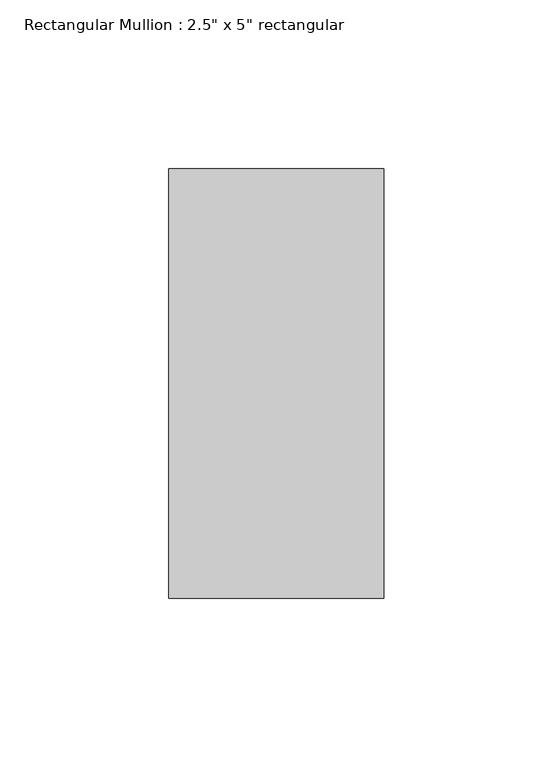
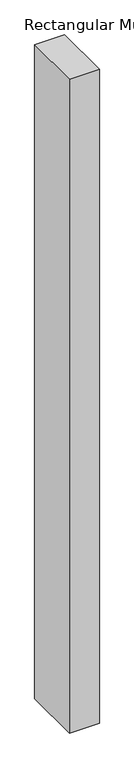
"""IFC4 building model written with IfcOpenShell, lengths in millimetres: member geometry."""

from ifc_helpers import new_model, si_unit, frame, origin, place, context, project, spatial, polyline, outline, extrude, source, transform, mapped, element, save


def member_ea8ac20a(model_context):
    return source(origin(), model_context, "Body", "SweptSolid", [
        extrude(outline(polyline([(0.0, 63.5), (0.0, -63.5), (-63.5, -63.5), (-63.5, 63.5), (0.0, 63.5)])), frame((0.0, 0.0, -1463.715679), z_axis=(0.0, 0.0, 1.0), x_axis=(1.0, 0.0, 0.0)), (0.0, 0.0, 1.0), 1463.715679),
    ])


if __name__ == "__main__":
    model = new_model("IFC4")
    model_context = context("Model", 3, world=origin())
    ifc_project = project(units=[si_unit("LENGTHUNIT", "METRE", prefix="MILLI")], contexts=[model_context])
    site = spatial("IfcSite", under=ifc_project)
    building = spatial("IfcBuilding", under=site)
    placement = place(None, origin())
    member_shape = member_ea8ac20a(model_context)
    element("IfcMember", 1, ObjectType="Rectangular Mullion : 2.5\" x 5\" rectangular", at=placement, inside=building, context=model_context, shape_type="MappedRepresentation", body=[
        mapped(member_shape, transform((0.0, 0.0, 0.0), x_axis=(1.0, 0.0, 0.0), y_axis=(0.0, 1.0, 0.0), z_axis=(0.0, 0.0, 1.0))),
    ])
    save(model, "model.ifc")

# Revit data of these elements
# Type "Rectangular Mullion : 2.5\" x 5\" rectangular"
#   built-in parameter 1007304 = 0.416667 (stored number, unit not read)
#   built-in parameter 1007301 = 0.104167 (stored number, unit not read)
#   built-in parameter 1007300 = 0.104167 (stored number, unit not read)
# Element 1 (IfcMember, "Rectangular Mullion : 2.5\" x 5\" rectangular")
#   Materials on its faces: "Aluminum"
# Materials
#   "Aluminum": class "Metal", colour RGB 247 247 247, transparency 0, Description = "Aluminum 6061", Cost = 0
